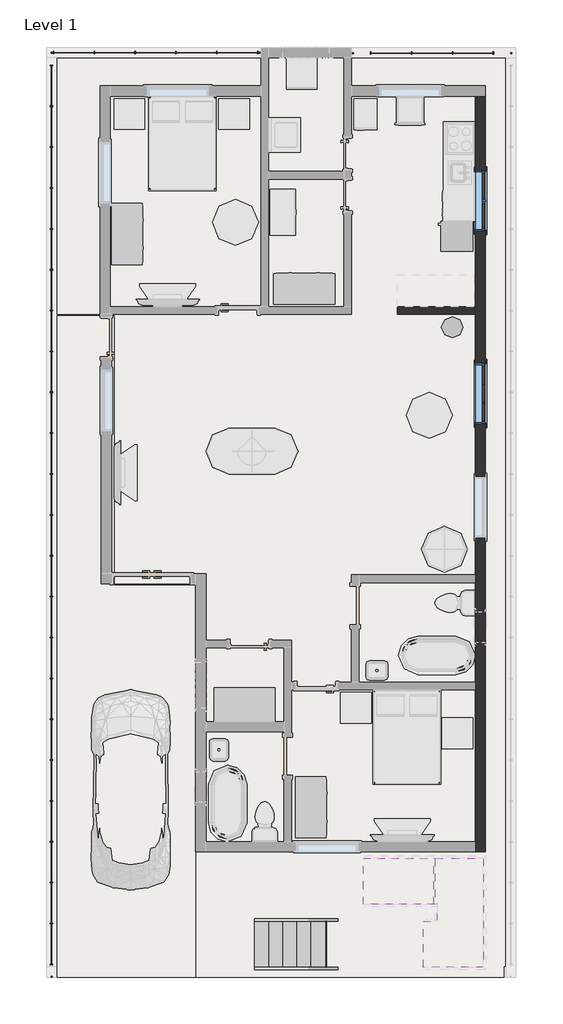
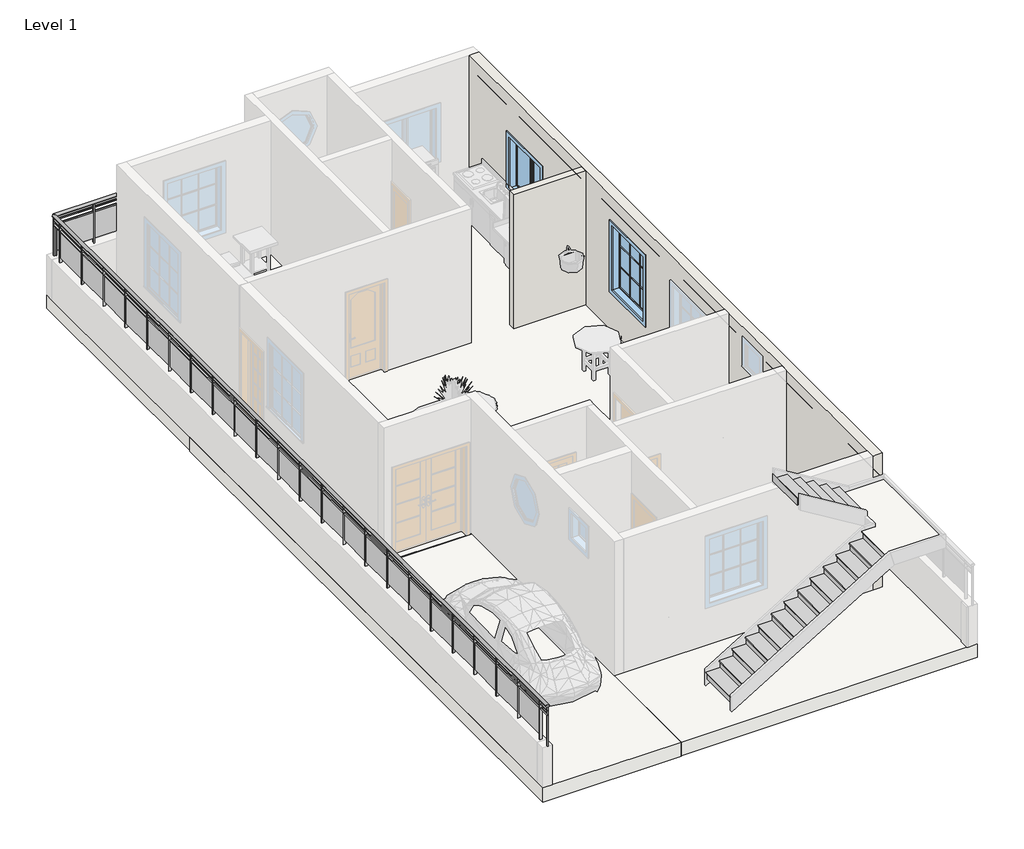
# One storey, part 2 of 3: 3 railings, 3 slabs, 2 stair flights, 2 walls, 2 windows.
"""IFC4 building model written with IfcOpenShell, lengths in millimetres."""

from ifc_helpers import new_model, si_unit, point, frame, origin, origin_with_axes, place, context, project, spatial, polyline, ellipse_curve, trimmed, outline, extrude, faceted_brep, transform, mapped, element, save
from ifc_brep_helpers import plane_surface, extruded_surface, advanced_brep
from components import non_monolithic_landing_d9a0f4c8, stair_flight_2c1cbba1, stair_flight_74d64587, window_cfa1ffdd, window_0862ab64

model = new_model("IFC4")

# Units and contexts
model_context = context("Model", 3, world=origin())
ifc_project = project(units=[si_unit("LENGTHUNIT", "METRE", prefix="MILLI")], contexts=[model_context])

# Site, building, storey
site = spatial("IfcSite", under=ifc_project)
building = spatial("IfcBuilding", under=site)
storey = spatial("IfcBuildingStorey", under=building, Name="Level 1", Elevation=0.0)

# Railings
placement = place(None, origin())
element("IfcRailing", 1, ObjectType="Glass Panel - Bottom Fill", at=placement, inside=storey, context=model_context, shape_type="SolidModel", body=[
    advanced_brep(
    [(-3535.608395, 15334.3151182, 1828.8), (-3535.608395, 15410.5151182, 1828.8), (-7675.808395, 15334.3151182, 1828.8), (-7675.808395, 15410.5151182, 1828.8)],
    [
        (0, 1, ellipse_curve(frame((-3535.608395, 15372.4151182, 1828.8), z_axis=(1.0, 0.0, 0.0), x_axis=(0.0, 1.0, 0.0)), 38.1, 28.575)),
        (1, 0, ellipse_curve(frame((-3535.608395, 15372.4151182, 1828.8), z_axis=(1.0, 0.0, 0.0), x_axis=(0.0, 1.0, 0.0)), 38.1, 28.575)),
        (2, 3, ellipse_curve(frame((-7675.808395, 15372.4151182, 1828.8), z_axis=(-1.0, 0.0, 0.0), x_axis=(0.0, 1.0, 0.0)), 38.1, 28.575)),
        (3, 2, ellipse_curve(frame((-7675.808395, 15372.4151182, 1828.8), z_axis=(-1.0, 0.0, 0.0), x_axis=(0.0, 1.0, 0.0)), 38.1, 28.575)),
        (0, 2),
        (3, 1),
    ],
    [
        plane_surface(frame((-3535.608395, 15372.4151182, 1828.8), z_axis=(1.0, 0.0, 0.0), x_axis=(0.0, -1.0, 0.0))),
        plane_surface(frame((-7675.808395, 15372.4151182, 1828.8), z_axis=(-1.0, 0.0, 0.0), x_axis=(0.0, -1.0, 0.0))),
        extruded_surface(trimmed(ellipse_curve(frame((-7675.808395, 15372.4151182, 1828.8), z_axis=(1.0, 0.0, 0.0), x_axis=(0.0, 1.0, 0.0)), 38.1, 28.575), [point((-7675.808395, 15334.3151182, 1828.8))], [point((-7675.808395, 15410.5151182, 1828.8))], True, "CARTESIAN"), (4140.2, 0.0, 0.0), 4140.2),
        extruded_surface(trimmed(ellipse_curve(frame((-7675.808395, 15372.4151182, 1828.8), z_axis=(1.0, 0.0, 0.0), x_axis=(0.0, 1.0, 0.0)), 38.1, 28.575), [point((-7675.808395, 15410.5151182, 1828.8))], [point((-7675.808395, 15334.3151182, 1828.8))], True, "CARTESIAN"), (4140.2, 0.0, 0.0), 4140.2),
    ],
    [
        (0, [[1, 2]]),
        (1, [[3, 4]]),
        (2, [[-1, 5, -4, 6]]),
        (3, [[-2, -6, -3, -5]]),
    ],
),
    extrude(outline(polyline([(-3535.608395, 15385.1151182), (-3535.608395, 15359.7151182), (-7675.808395, 15359.7151182), (-7675.808395, 15385.1151182), (-3535.608395, 15385.1151182)])), frame((0.0, 0.0, 1714.5), z_axis=(0.0, 0.0, 1.0), x_axis=(1.0, 0.0, 0.0)), (0.0, 0.0, 1.0), 25.4),
    extrude(outline(polyline([(-3535.608395, 15385.1151182), (-3535.608395, 15359.7151182), (-7675.808395, 15359.7151182), (-7675.808395, 15385.1151182), (-3535.608395, 15385.1151182)])), frame((0.0, 0.0, 1612.9), z_axis=(0.0, 0.0, 1.0), x_axis=(1.0, 0.0, 0.0)), (0.0, 0.0, 1.0), 25.4),
    extrude(outline(polyline([(-7631.358395, 15397.8151182), (-7631.358395, 15347.0151182), (-7644.058395, 15347.0151182), (-7644.058395, 15397.8151182), (-7631.358395, 15397.8151182)])), frame((0.0, 0.0, 914.4), z_axis=(0.0, 0.0, 1.0), x_axis=(1.0, 0.0, 0.0)), (0.0, 0.0, 1.0), 885.6788223),
    extrude(outline(polyline([(-6824.908395, 15365.8799612), (-7637.708395, 15365.8799612), (-7637.708395, 15372.2299612), (-6824.908395, 15372.2299612), (-6824.908395, 15365.8799612)])), frame((0.0, 0.0, 1016.0), z_axis=(0.0, 0.0, 1.0), x_axis=(1.0, 0.0, 0.0)), (0.0, 0.0, 1.0), 596.9),
    extrude(outline(polyline([(-6818.558395, 15397.8151182), (-6818.558395, 15347.0151182), (-6831.258395, 15347.0151182), (-6831.258395, 15397.8151182), (-6818.558395, 15397.8151182)])), frame((0.0, 0.0, 914.4), z_axis=(0.0, 0.0, 1.0), x_axis=(1.0, 0.0, 0.0)), (0.0, 0.0, 1.0), 885.6788223),
    extrude(outline(polyline([(-6012.108395, 15365.8799612), (-6824.908395, 15365.8799612), (-6824.908395, 15372.2299612), (-6012.108395, 15372.2299612), (-6012.108395, 15365.8799612)])), frame((0.0, 0.0, 1016.0), z_axis=(0.0, 0.0, 1.0), x_axis=(1.0, 0.0, 0.0)), (0.0, 0.0, 1.0), 596.9),
    extrude(outline(polyline([(-6005.758395, 15397.8151182), (-6005.758395, 15347.0151182), (-6018.458395, 15347.0151182), (-6018.458395, 15397.8151182), (-6005.758395, 15397.8151182)])), frame((0.0, 0.0, 914.4), z_axis=(0.0, 0.0, 1.0), x_axis=(1.0, 0.0, 0.0)), (0.0, 0.0, 1.0), 885.6788223),
    extrude(outline(polyline([(-5199.308395, 15365.8799612), (-6012.108395, 15365.8799612), (-6012.108395, 15372.2299612), (-5199.308395, 15372.2299612), (-5199.308395, 15365.8799612)])), frame((0.0, 0.0, 1016.0), z_axis=(0.0, 0.0, 1.0), x_axis=(1.0, 0.0, 0.0)), (0.0, 0.0, 1.0), 596.9),
    extrude(outline(polyline([(-5192.958395, 15397.8151182), (-5192.958395, 15347.0151182), (-5205.658395, 15347.0151182), (-5205.658395, 15397.8151182), (-5192.958395, 15397.8151182)])), frame((0.0, 0.0, 914.4), z_axis=(0.0, 0.0, 1.0), x_axis=(1.0, 0.0, 0.0)), (0.0, 0.0, 1.0), 885.6788223),
    extrude(outline(polyline([(-4386.508395, 15365.8799612), (-5199.308395, 15365.8799612), (-5199.308395, 15372.2299612), (-4386.508395, 15372.2299612), (-4386.508395, 15365.8799612)])), frame((0.0, 0.0, 1016.0), z_axis=(0.0, 0.0, 1.0), x_axis=(1.0, 0.0, 0.0)), (0.0, 0.0, 1.0), 596.9),
    extrude(outline(polyline([(-4380.158395, 15397.8151182), (-4380.158395, 15347.0151182), (-4392.858395, 15347.0151182), (-4392.858395, 15397.8151182), (-4380.158395, 15397.8151182)])), frame((0.0, 0.0, 914.4), z_axis=(0.0, 0.0, 1.0), x_axis=(1.0, 0.0, 0.0)), (0.0, 0.0, 1.0), 885.6788223),
    extrude(outline(polyline([(-3573.708395, 15365.8799612), (-4386.508395, 15365.8799612), (-4386.508395, 15372.2299612), (-3573.708395, 15372.2299612), (-3573.708395, 15365.8799612)])), frame((0.0, 0.0, 1016.0), z_axis=(0.0, 0.0, 1.0), x_axis=(1.0, 0.0, 0.0)), (0.0, 0.0, 1.0), 596.9),
    extrude(outline(polyline([(-3567.358395, 15397.8151182), (-3567.358395, 15347.0151182), (-3580.058395, 15347.0151182), (-3580.058395, 15397.8151182), (-3567.358395, 15397.8151182)])), frame((0.0, 0.0, 914.4), z_axis=(0.0, 0.0, 1.0), x_axis=(1.0, 0.0, 0.0)), (0.0, 0.0, 1.0), 885.6788223),
    extrude(outline(polyline([(-7663.108395, 15381.9401182), (-7663.108395, 15362.8901182), (-7682.158395, 15362.8901182), (-7682.158395, 15381.9401182), (-7663.108395, 15381.9401182)])), frame((0.0, 0.0, 914.4), z_axis=(0.0, 0.0, 1.0), x_axis=(1.0, 0.0, 0.0)), (0.0, 0.0, 1.0), 885.6788223),
    extrude(outline(polyline([(-3529.258395, 15381.9401182), (-3529.258395, 15362.8901182), (-3548.308395, 15362.8901182), (-3548.308395, 15381.9401182), (-3529.258395, 15381.9401182)])), frame((0.0, 0.0, 914.4), z_axis=(0.0, 0.0, 1.0), x_axis=(1.0, 0.0, 0.0)), (0.0, 0.0, 1.0), 885.6788223),
])
element("IfcRailing", 2, ObjectType="Glass Panel - Bottom Fill", at=placement, inside=storey, context=model_context, shape_type="SolidModel", body=[
    advanced_brep(
    [(-7637.708395, 15372.4151182, 1828.8), (-7713.908395, 15372.4151182, 1828.8), (-7637.708395, -3017.1848818, 1828.8), (-7713.908395, -3017.1848818, 1828.8)],
    [
        (0, 1, ellipse_curve(frame((-7675.808395, 15372.4151182, 1828.8), z_axis=(0.0, 1.0, 0.0), x_axis=(-1.0, 0.0, 0.0)), 38.1, 28.575)),
        (1, 0, ellipse_curve(frame((-7675.808395, 15372.4151182, 1828.8), z_axis=(0.0, 1.0, 0.0), x_axis=(-1.0, 0.0, 0.0)), 38.1, 28.575)),
        (2, 3, ellipse_curve(frame((-7675.808395, -3017.1848818, 1828.8), z_axis=(0.0, -1.0, 0.0), x_axis=(-1.0, 0.0, 0.0)), 38.1, 28.575)),
        (3, 2, ellipse_curve(frame((-7675.808395, -3017.1848818, 1828.8), z_axis=(0.0, -1.0, 0.0), x_axis=(-1.0, 0.0, 0.0)), 38.1, 28.575)),
        (0, 2),
        (3, 1),
    ],
    [
        plane_surface(frame((-7675.808395, 15372.4151182, 1828.8), z_axis=(0.0, 1.0, 0.0), x_axis=(0.0, 0.0, -1.0))),
        plane_surface(frame((-7675.808395, -3017.1848818, 1828.8), z_axis=(0.0, -1.0, 0.0), x_axis=(0.0, 0.0, -1.0))),
        extruded_surface(trimmed(ellipse_curve(frame((-7675.808395, -3017.1848818, 1828.8), z_axis=(0.0, 1.0, 0.0), x_axis=(-1.0, 0.0, 0.0)), 38.1, 28.575), [point((-7637.708395, -3017.1848818, 1828.8))], [point((-7713.908395, -3017.1848818, 1828.8))], True, "CARTESIAN"), (0.0, 18389.6, 0.0), 18389.6),
        extruded_surface(trimmed(ellipse_curve(frame((-7675.808395, -3017.1848818, 1828.8), z_axis=(0.0, 1.0, 0.0), x_axis=(-1.0, 0.0, 0.0)), 38.1, 28.575), [point((-7713.908395, -3017.1848818, 1828.8))], [point((-7637.708395, -3017.1848818, 1828.8))], True, "CARTESIAN"), (0.0, 18389.6, 0.0), 18389.6),
    ],
    [
        (0, [[1, 2]]),
        (1, [[3, 4]]),
        (2, [[-1, 5, -4, 6]]),
        (3, [[-2, -6, -3, -5]]),
    ],
),
    extrude(outline(polyline([(-7688.508395, 15372.4151182), (-7663.108395, 15372.4151182), (-7663.108395, -3017.1848818), (-7688.508395, -3017.1848818), (-7688.508395, 15372.4151182)])), frame((0.0, 0.0, 1714.5), z_axis=(0.0, 0.0, 1.0), x_axis=(1.0, 0.0, 0.0)), (0.0, 0.0, 1.0), 25.4),
    extrude(outline(polyline([(-7688.508395, 15372.4151182), (-7663.108395, 15372.4151182), (-7663.108395, -3017.1848818), (-7688.508395, -3017.1848818), (-7688.508395, 15372.4151182)])), frame((0.0, 0.0, 1612.9), z_axis=(0.0, 0.0, 1.0), x_axis=(1.0, 0.0, 0.0)), (0.0, 0.0, 1.0), 25.4),
    extrude(outline(polyline([(-7650.408395, -2756.8348818), (-7650.408395, -2769.5348818), (-7701.208395, -2769.5348818), (-7701.208395, -2756.8348818), (-7650.408395, -2756.8348818)])), frame((0.0, 0.0, 914.4), z_axis=(0.0, 0.0, 1.0), x_axis=(1.0, 0.0, 0.0)), (0.0, 0.0, 1.0), 885.6788223),
    extrude(outline(polyline([(-7682.343552, -1950.3848818), (-7675.993552, -1950.3848818), (-7675.993552, -2763.1848818), (-7682.343552, -2763.1848818), (-7682.343552, -1950.3848818)])), frame((0.0, 0.0, 1016.0), z_axis=(0.0, 0.0, 1.0), x_axis=(1.0, 0.0, 0.0)), (0.0, 0.0, 1.0), 596.9),
    extrude(outline(polyline([(-7650.408395, -1944.0348818), (-7650.408395, -1956.7348818), (-7701.208395, -1956.7348818), (-7701.208395, -1944.0348818), (-7650.408395, -1944.0348818)])), frame((0.0, 0.0, 914.4), z_axis=(0.0, 0.0, 1.0), x_axis=(1.0, 0.0, 0.0)), (0.0, 0.0, 1.0), 885.6788223),
    extrude(outline(polyline([(-7682.343552, -1137.5848818), (-7675.993552, -1137.5848818), (-7675.993552, -1950.3848818), (-7682.343552, -1950.3848818), (-7682.343552, -1137.5848818)])), frame((0.0, 0.0, 1016.0), z_axis=(0.0, 0.0, 1.0), x_axis=(1.0, 0.0, 0.0)), (0.0, 0.0, 1.0), 596.9),
    extrude(outline(polyline([(-7650.408395, -1131.2348818), (-7650.408395, -1143.9348818), (-7701.208395, -1143.9348818), (-7701.208395, -1131.2348818), (-7650.408395, -1131.2348818)])), frame((0.0, 0.0, 914.4), z_axis=(0.0, 0.0, 1.0), x_axis=(1.0, 0.0, 0.0)), (0.0, 0.0, 1.0), 885.6788223),
    extrude(outline(polyline([(-7682.343552, -324.7848818), (-7675.993552, -324.7848818), (-7675.993552, -1137.5848818), (-7682.343552, -1137.5848818), (-7682.343552, -324.7848818)])), frame((0.0, 0.0, 1016.0), z_axis=(0.0, 0.0, 1.0), x_axis=(1.0, 0.0, 0.0)), (0.0, 0.0, 1.0), 596.9),
    extrude(outline(polyline([(-7650.408395, -318.4348818), (-7650.408395, -331.1348818), (-7701.208395, -331.1348818), (-7701.208395, -318.4348818), (-7650.408395, -318.4348818)])), frame((0.0, 0.0, 914.4), z_axis=(0.0, 0.0, 1.0), x_axis=(1.0, 0.0, 0.0)), (0.0, 0.0, 1.0), 885.6788223),
    extrude(outline(polyline([(-7682.343552, 488.0151182), (-7675.993552, 488.0151182), (-7675.993552, -324.7848818), (-7682.343552, -324.7848818), (-7682.343552, 488.0151182)])), frame((0.0, 0.0, 1016.0), z_axis=(0.0, 0.0, 1.0), x_axis=(1.0, 0.0, 0.0)), (0.0, 0.0, 1.0), 596.9),
    extrude(outline(polyline([(-7650.408395, 494.3651182), (-7650.408395, 481.6651182), (-7701.208395, 481.6651182), (-7701.208395, 494.3651182), (-7650.408395, 494.3651182)])), frame((0.0, 0.0, 914.4), z_axis=(0.0, 0.0, 1.0), x_axis=(1.0, 0.0, 0.0)), (0.0, 0.0, 1.0), 885.6788223),
    extrude(outline(polyline([(-7682.343552, 1300.8151182), (-7675.993552, 1300.8151182), (-7675.993552, 488.0151182), (-7682.343552, 488.0151182), (-7682.343552, 1300.8151182)])), frame((0.0, 0.0, 1016.0), z_axis=(0.0, 0.0, 1.0), x_axis=(1.0, 0.0, 0.0)), (0.0, 0.0, 1.0), 596.9),
    extrude(outline(polyline([(-7650.408395, 1307.1651182), (-7650.408395, 1294.4651182), (-7701.208395, 1294.4651182), (-7701.208395, 1307.1651182), (-7650.408395, 1307.1651182)])), frame((0.0, 0.0, 914.4), z_axis=(0.0, 0.0, 1.0), x_axis=(1.0, 0.0, 0.0)), (0.0, 0.0, 1.0), 885.6788223),
    extrude(outline(polyline([(-7682.343552, 2113.6151182), (-7675.993552, 2113.6151182), (-7675.993552, 1300.8151182), (-7682.343552, 1300.8151182), (-7682.343552, 2113.6151182)])), frame((0.0, 0.0, 1016.0), z_axis=(0.0, 0.0, 1.0), x_axis=(1.0, 0.0, 0.0)), (0.0, 0.0, 1.0), 596.9),
    extrude(outline(polyline([(-7650.408395, 2119.9651182), (-7650.408395, 2107.2651182), (-7701.208395, 2107.2651182), (-7701.208395, 2119.9651182), (-7650.408395, 2119.9651182)])), frame((0.0, 0.0, 914.4), z_axis=(0.0, 0.0, 1.0), x_axis=(1.0, 0.0, 0.0)), (0.0, 0.0, 1.0), 885.6788223),
    extrude(outline(polyline([(-7682.343552, 2926.4151182), (-7675.993552, 2926.4151182), (-7675.993552, 2113.6151182), (-7682.343552, 2113.6151182), (-7682.343552, 2926.4151182)])), frame((0.0, 0.0, 1016.0), z_axis=(0.0, 0.0, 1.0), x_axis=(1.0, 0.0, 0.0)), (0.0, 0.0, 1.0), 596.9),
    extrude(outline(polyline([(-7650.408395, 2932.7651182), (-7650.408395, 2920.0651182), (-7701.208395, 2920.0651182), (-7701.208395, 2932.7651182), (-7650.408395, 2932.7651182)])), frame((0.0, 0.0, 914.4), z_axis=(0.0, 0.0, 1.0), x_axis=(1.0, 0.0, 0.0)), (0.0, 0.0, 1.0), 885.6788223),
    extrude(outline(polyline([(-7682.343552, 3739.2151182), (-7675.993552, 3739.2151182), (-7675.993552, 2926.4151182), (-7682.343552, 2926.4151182), (-7682.343552, 3739.2151182)])), frame((0.0, 0.0, 1016.0), z_axis=(0.0, 0.0, 1.0), x_axis=(1.0, 0.0, 0.0)), (0.0, 0.0, 1.0), 596.9),
    extrude(outline(polyline([(-7650.408395, 3745.5651182), (-7650.408395, 3732.8651182), (-7701.208395, 3732.8651182), (-7701.208395, 3745.5651182), (-7650.408395, 3745.5651182)])), frame((0.0, 0.0, 914.4), z_axis=(0.0, 0.0, 1.0), x_axis=(1.0, 0.0, 0.0)), (0.0, 0.0, 1.0), 885.6788223),
    extrude(outline(polyline([(-7682.343552, 4552.0151182), (-7675.993552, 4552.0151182), (-7675.993552, 3739.2151182), (-7682.343552, 3739.2151182), (-7682.343552, 4552.0151182)])), frame((0.0, 0.0, 1016.0), z_axis=(0.0, 0.0, 1.0), x_axis=(1.0, 0.0, 0.0)), (0.0, 0.0, 1.0), 596.9),
    extrude(outline(polyline([(-7650.408395, 4558.3651182), (-7650.408395, 4545.6651182), (-7701.208395, 4545.6651182), (-7701.208395, 4558.3651182), (-7650.408395, 4558.3651182)])), frame((0.0, 0.0, 914.4), z_axis=(0.0, 0.0, 1.0), x_axis=(1.0, 0.0, 0.0)), (0.0, 0.0, 1.0), 885.6788223),
    extrude(outline(polyline([(-7682.343552, 5364.8151182), (-7675.993552, 5364.8151182), (-7675.993552, 4552.0151182), (-7682.343552, 4552.0151182), (-7682.343552, 5364.8151182)])), frame((0.0, 0.0, 1016.0), z_axis=(0.0, 0.0, 1.0), x_axis=(1.0, 0.0, 0.0)), (0.0, 0.0, 1.0), 596.9),
    extrude(outline(polyline([(-7650.408395, 5371.1651182), (-7650.408395, 5358.4651182), (-7701.208395, 5358.4651182), (-7701.208395, 5371.1651182), (-7650.408395, 5371.1651182)])), frame((0.0, 0.0, 914.4), z_axis=(0.0, 0.0, 1.0), x_axis=(1.0, 0.0, 0.0)), (0.0, 0.0, 1.0), 885.6788223),
    extrude(outline(polyline([(-7682.343552, 6177.6151182), (-7675.993552, 6177.6151182), (-7675.993552, 5364.8151182), (-7682.343552, 5364.8151182), (-7682.343552, 6177.6151182)])), frame((0.0, 0.0, 1016.0), z_axis=(0.0, 0.0, 1.0), x_axis=(1.0, 0.0, 0.0)), (0.0, 0.0, 1.0), 596.9),
    extrude(outline(polyline([(-7650.408395, 6183.9651182), (-7650.408395, 6171.2651182), (-7701.208395, 6171.2651182), (-7701.208395, 6183.9651182), (-7650.408395, 6183.9651182)])), frame((0.0, 0.0, 914.4), z_axis=(0.0, 0.0, 1.0), x_axis=(1.0, 0.0, 0.0)), (0.0, 0.0, 1.0), 885.6788223),
    extrude(outline(polyline([(-7682.343552, 6990.4151182), (-7675.993552, 6990.4151182), (-7675.993552, 6177.6151182), (-7682.343552, 6177.6151182), (-7682.343552, 6990.4151182)])), frame((0.0, 0.0, 1016.0), z_axis=(0.0, 0.0, 1.0), x_axis=(1.0, 0.0, 0.0)), (0.0, 0.0, 1.0), 596.9),
    extrude(outline(polyline([(-7650.408395, 6996.7651182), (-7650.408395, 6984.0651182), (-7701.208395, 6984.0651182), (-7701.208395, 6996.7651182), (-7650.408395, 6996.7651182)])), frame((0.0, 0.0, 914.4), z_axis=(0.0, 0.0, 1.0), x_axis=(1.0, 0.0, 0.0)), (0.0, 0.0, 1.0), 885.6788223),
    extrude(outline(polyline([(-7682.343552, 7803.2151182), (-7675.993552, 7803.2151182), (-7675.993552, 6990.4151182), (-7682.343552, 6990.4151182), (-7682.343552, 7803.2151182)])), frame((0.0, 0.0, 1016.0), z_axis=(0.0, 0.0, 1.0), x_axis=(1.0, 0.0, 0.0)), (0.0, 0.0, 1.0), 596.9),
    extrude(outline(polyline([(-7650.408395, 7809.5651182), (-7650.408395, 7796.8651182), (-7701.208395, 7796.8651182), (-7701.208395, 7809.5651182), (-7650.408395, 7809.5651182)])), frame((0.0, 0.0, 914.4), z_axis=(0.0, 0.0, 1.0), x_axis=(1.0, 0.0, 0.0)), (0.0, 0.0, 1.0), 885.6788223),
    extrude(outline(polyline([(-7682.343552, 8616.0151182), (-7675.993552, 8616.0151182), (-7675.993552, 7803.2151182), (-7682.343552, 7803.2151182), (-7682.343552, 8616.0151182)])), frame((0.0, 0.0, 1016.0), z_axis=(0.0, 0.0, 1.0), x_axis=(1.0, 0.0, 0.0)), (0.0, 0.0, 1.0), 596.9),
    extrude(outline(polyline([(-7650.408395, 8622.3651182), (-7650.408395, 8609.6651182), (-7701.208395, 8609.6651182), (-7701.208395, 8622.3651182), (-7650.408395, 8622.3651182)])), frame((0.0, 0.0, 914.4), z_axis=(0.0, 0.0, 1.0), x_axis=(1.0, 0.0, 0.0)), (0.0, 0.0, 1.0), 885.6788223),
    extrude(outline(polyline([(-7682.343552, 9428.8151182), (-7675.993552, 9428.8151182), (-7675.993552, 8616.0151182), (-7682.343552, 8616.0151182), (-7682.343552, 9428.8151182)])), frame((0.0, 0.0, 1016.0), z_axis=(0.0, 0.0, 1.0), x_axis=(1.0, 0.0, 0.0)), (0.0, 0.0, 1.0), 596.9),
    extrude(outline(polyline([(-7650.408395, 9435.1651182), (-7650.408395, 9422.4651182), (-7701.208395, 9422.4651182), (-7701.208395, 9435.1651182), (-7650.408395, 9435.1651182)])), frame((0.0, 0.0, 914.4), z_axis=(0.0, 0.0, 1.0), x_axis=(1.0, 0.0, 0.0)), (0.0, 0.0, 1.0), 885.6788223),
    extrude(outline(polyline([(-7682.343552, 10241.6151182), (-7675.993552, 10241.6151182), (-7675.993552, 9428.8151182), (-7682.343552, 9428.8151182), (-7682.343552, 10241.6151182)])), frame((0.0, 0.0, 1016.0), z_axis=(0.0, 0.0, 1.0), x_axis=(1.0, 0.0, 0.0)), (0.0, 0.0, 1.0), 596.9),
    extrude(outline(polyline([(-7650.408395, 10247.9651182), (-7650.408395, 10235.2651182), (-7701.208395, 10235.2651182), (-7701.208395, 10247.9651182), (-7650.408395, 10247.9651182)])), frame((0.0, 0.0, 914.4), z_axis=(0.0, 0.0, 1.0), x_axis=(1.0, 0.0, 0.0)), (0.0, 0.0, 1.0), 885.6788223),
    extrude(outline(polyline([(-7682.343552, 11054.4151182), (-7675.993552, 11054.4151182), (-7675.993552, 10241.6151182), (-7682.343552, 10241.6151182), (-7682.343552, 11054.4151182)])), frame((0.0, 0.0, 1016.0), z_axis=(0.0, 0.0, 1.0), x_axis=(1.0, 0.0, 0.0)), (0.0, 0.0, 1.0), 596.9),
    extrude(outline(polyline([(-7650.408395, 11060.7651182), (-7650.408395, 11048.0651182), (-7701.208395, 11048.0651182), (-7701.208395, 11060.7651182), (-7650.408395, 11060.7651182)])), frame((0.0, 0.0, 914.4), z_axis=(0.0, 0.0, 1.0), x_axis=(1.0, 0.0, 0.0)), (0.0, 0.0, 1.0), 885.6788223),
    extrude(outline(polyline([(-7682.343552, 11867.2151182), (-7675.993552, 11867.2151182), (-7675.993552, 11054.4151182), (-7682.343552, 11054.4151182), (-7682.343552, 11867.2151182)])), frame((0.0, 0.0, 1016.0), z_axis=(0.0, 0.0, 1.0), x_axis=(1.0, 0.0, 0.0)), (0.0, 0.0, 1.0), 596.9),
    extrude(outline(polyline([(-7650.408395, 11873.5651182), (-7650.408395, 11860.8651182), (-7701.208395, 11860.8651182), (-7701.208395, 11873.5651182), (-7650.408395, 11873.5651182)])), frame((0.0, 0.0, 914.4), z_axis=(0.0, 0.0, 1.0), x_axis=(1.0, 0.0, 0.0)), (0.0, 0.0, 1.0), 885.6788223),
    extrude(outline(polyline([(-7682.343552, 12680.0151182), (-7675.993552, 12680.0151182), (-7675.993552, 11867.2151182), (-7682.343552, 11867.2151182), (-7682.343552, 12680.0151182)])), frame((0.0, 0.0, 1016.0), z_axis=(0.0, 0.0, 1.0), x_axis=(1.0, 0.0, 0.0)), (0.0, 0.0, 1.0), 596.9),
    extrude(outline(polyline([(-7650.408395, 12686.3651182), (-7650.408395, 12673.6651182), (-7701.208395, 12673.6651182), (-7701.208395, 12686.3651182), (-7650.408395, 12686.3651182)])), frame((0.0, 0.0, 914.4), z_axis=(0.0, 0.0, 1.0), x_axis=(1.0, 0.0, 0.0)), (0.0, 0.0, 1.0), 885.6788223),
    extrude(outline(polyline([(-7682.343552, 13492.8151182), (-7675.993552, 13492.8151182), (-7675.993552, 12680.0151182), (-7682.343552, 12680.0151182), (-7682.343552, 13492.8151182)])), frame((0.0, 0.0, 1016.0), z_axis=(0.0, 0.0, 1.0), x_axis=(1.0, 0.0, 0.0)), (0.0, 0.0, 1.0), 596.9),
    extrude(outline(polyline([(-7650.408395, 13499.1651182), (-7650.408395, 13486.4651182), (-7701.208395, 13486.4651182), (-7701.208395, 13499.1651182), (-7650.408395, 13499.1651182)])), frame((0.0, 0.0, 914.4), z_axis=(0.0, 0.0, 1.0), x_axis=(1.0, 0.0, 0.0)), (0.0, 0.0, 1.0), 885.6788223),
    extrude(outline(polyline([(-7682.343552, 14305.6151182), (-7675.993552, 14305.6151182), (-7675.993552, 13492.8151182), (-7682.343552, 13492.8151182), (-7682.343552, 14305.6151182)])), frame((0.0, 0.0, 1016.0), z_axis=(0.0, 0.0, 1.0), x_axis=(1.0, 0.0, 0.0)), (0.0, 0.0, 1.0), 596.9),
    extrude(outline(polyline([(-7650.408395, 14311.9651182), (-7650.408395, 14299.2651182), (-7701.208395, 14299.2651182), (-7701.208395, 14311.9651182), (-7650.408395, 14311.9651182)])), frame((0.0, 0.0, 914.4), z_axis=(0.0, 0.0, 1.0), x_axis=(1.0, 0.0, 0.0)), (0.0, 0.0, 1.0), 885.6788223),
    extrude(outline(polyline([(-7682.343552, 15118.4151182), (-7675.993552, 15118.4151182), (-7675.993552, 14305.6151182), (-7682.343552, 14305.6151182), (-7682.343552, 15118.4151182)])), frame((0.0, 0.0, 1016.0), z_axis=(0.0, 0.0, 1.0), x_axis=(1.0, 0.0, 0.0)), (0.0, 0.0, 1.0), 596.9),
    extrude(outline(polyline([(-7650.408395, 15124.7651182), (-7650.408395, 15112.0651182), (-7701.208395, 15112.0651182), (-7701.208395, 15124.7651182), (-7650.408395, 15124.7651182)])), frame((0.0, 0.0, 914.4), z_axis=(0.0, 0.0, 1.0), x_axis=(1.0, 0.0, 0.0)), (0.0, 0.0, 1.0), 885.6788223),
    extrude(outline(polyline([(-7666.283395, -3004.4848818), (-7666.283395, -3023.5348818), (-7685.333395, -3023.5348818), (-7685.333395, -3004.4848818), (-7666.283395, -3004.4848818)])), frame((0.0, 0.0, 914.4), z_axis=(0.0, 0.0, 1.0), x_axis=(1.0, 0.0, 0.0)), (0.0, 0.0, 1.0), 885.6788223),
    extrude(outline(polyline([(-7666.283395, 15378.7651182), (-7666.283395, 15359.7151182), (-7685.333395, 15359.7151182), (-7685.333395, 15378.7651182), (-7666.283395, 15378.7651182)])), frame((0.0, 0.0, 914.4), z_axis=(0.0, 0.0, 1.0), x_axis=(1.0, 0.0, 0.0)), (0.0, 0.0, 1.0), 885.6788223),
])
element("IfcRailing", 3, ObjectType="Glass Panel - Bottom Fill", at=placement, inside=storey, context=model_context, shape_type="SolidModel", body=[
    advanced_brep(
    [(1477.716605, 15324.7901182, 1828.8), (1477.716605, 15400.9901182, 1828.8), (-1681.408395, 15324.7901182, 1828.8), (-1681.408395, 15400.9901182, 1828.8)],
    [
        (0, 1, ellipse_curve(frame((1477.716605, 15362.8901182, 1828.8), z_axis=(1.0, 0.0, 0.0), x_axis=(0.0, 1.0, 0.0)), 38.1, 28.575)),
        (1, 0, ellipse_curve(frame((1477.716605, 15362.8901182, 1828.8), z_axis=(1.0, 0.0, 0.0), x_axis=(0.0, 1.0, 0.0)), 38.1, 28.575)),
        (2, 3, ellipse_curve(frame((-1681.408395, 15362.8901182, 1828.8), z_axis=(-1.0, 0.0, 0.0), x_axis=(0.0, 1.0, 0.0)), 38.1, 28.575)),
        (3, 2, ellipse_curve(frame((-1681.408395, 15362.8901182, 1828.8), z_axis=(-1.0, 0.0, 0.0), x_axis=(0.0, 1.0, 0.0)), 38.1, 28.575)),
        (0, 2),
        (3, 1),
    ],
    [
        plane_surface(frame((1477.716605, 15362.8901182, 1828.8), z_axis=(1.0, 0.0, 0.0), x_axis=(0.0, -1.0, 0.0))),
        plane_surface(frame((-1681.408395, 15362.8901182, 1828.8), z_axis=(-1.0, 0.0, 0.0), x_axis=(0.0, -1.0, 0.0))),
        extruded_surface(trimmed(ellipse_curve(frame((-1681.408395, 15362.8901182, 1828.8), z_axis=(1.0, 0.0, 0.0), x_axis=(0.0, 1.0, 0.0)), 38.1, 28.575), [point((-1681.408395, 15324.7901182, 1828.8))], [point((-1681.408395, 15400.9901182, 1828.8))], True, "CARTESIAN"), (3159.125, 0.0, 0.0), 3159.125),
        extruded_surface(trimmed(ellipse_curve(frame((-1681.408395, 15362.8901182, 1828.8), z_axis=(1.0, 0.0, 0.0), x_axis=(0.0, 1.0, 0.0)), 38.1, 28.575), [point((-1681.408395, 15400.9901182, 1828.8))], [point((-1681.408395, 15324.7901182, 1828.8))], True, "CARTESIAN"), (3159.125, 0.0, 0.0), 3159.125),
    ],
    [
        (0, [[1, 2]]),
        (1, [[3, 4]]),
        (2, [[-1, 5, -4, 6]]),
        (3, [[-2, -6, -3, -5]]),
    ],
),
    extrude(outline(polyline([(1477.716605, 15375.5901182), (1477.716605, 15350.1901182), (-1681.408395, 15350.1901182), (-1681.408395, 15375.5901182), (1477.716605, 15375.5901182)])), frame((0.0, 0.0, 1714.5), z_axis=(0.0, 0.0, 1.0), x_axis=(1.0, 0.0, 0.0)), (0.0, 0.0, 1.0), 25.4),
    extrude(outline(polyline([(1477.716605, 15375.5901182), (1477.716605, 15350.1901182), (-1681.408395, 15350.1901182), (-1681.408395, 15375.5901182), (1477.716605, 15375.5901182)])), frame((0.0, 0.0, 1612.9), z_axis=(0.0, 0.0, 1.0), x_axis=(1.0, 0.0, 0.0)), (0.0, 0.0, 1.0), 25.4),
    extrude(outline(polyline([(-1314.695895, 15388.2901182), (-1314.695895, 15337.4901182), (-1327.395895, 15337.4901182), (-1327.395895, 15388.2901182), (-1314.695895, 15388.2901182)])), frame((0.0, 0.0, 914.4), z_axis=(0.0, 0.0, 1.0), x_axis=(1.0, 0.0, 0.0)), (0.0, 0.0, 1.0), 885.6788223),
    extrude(outline(polyline([(-508.245895, 15356.3549612), (-1321.045895, 15356.3549612), (-1321.045895, 15362.7049612), (-508.245895, 15362.7049612), (-508.245895, 15356.3549612)])), frame((0.0, 0.0, 1016.0), z_axis=(0.0, 0.0, 1.0), x_axis=(1.0, 0.0, 0.0)), (0.0, 0.0, 1.0), 596.9),
    extrude(outline(polyline([(-501.895895, 15388.2901182), (-501.895895, 15337.4901182), (-514.595895, 15337.4901182), (-514.595895, 15388.2901182), (-501.895895, 15388.2901182)])), frame((0.0, 0.0, 914.4), z_axis=(0.0, 0.0, 1.0), x_axis=(1.0, 0.0, 0.0)), (0.0, 0.0, 1.0), 885.6788223),
    extrude(outline(polyline([(304.554105, 15356.3549612), (-508.245895, 15356.3549612), (-508.245895, 15362.7049612), (304.554105, 15362.7049612), (304.554105, 15356.3549612)])), frame((0.0, 0.0, 1016.0), z_axis=(0.0, 0.0, 1.0), x_axis=(1.0, 0.0, 0.0)), (0.0, 0.0, 1.0), 596.9),
    extrude(outline(polyline([(310.904105, 15388.2901182), (310.904105, 15337.4901182), (298.204105, 15337.4901182), (298.204105, 15388.2901182), (310.904105, 15388.2901182)])), frame((0.0, 0.0, 914.4), z_axis=(0.0, 0.0, 1.0), x_axis=(1.0, 0.0, 0.0)), (0.0, 0.0, 1.0), 885.6788223),
    extrude(outline(polyline([(1117.354105, 15356.3549612), (304.554105, 15356.3549612), (304.554105, 15362.7049612), (1117.354105, 15362.7049612), (1117.354105, 15356.3549612)])), frame((0.0, 0.0, 1016.0), z_axis=(0.0, 0.0, 1.0), x_axis=(1.0, 0.0, 0.0)), (0.0, 0.0, 1.0), 596.9),
    extrude(outline(polyline([(1123.704105, 15388.2901182), (1123.704105, 15337.4901182), (1111.004105, 15337.4901182), (1111.004105, 15388.2901182), (1123.704105, 15388.2901182)])), frame((0.0, 0.0, 914.4), z_axis=(0.0, 0.0, 1.0), x_axis=(1.0, 0.0, 0.0)), (0.0, 0.0, 1.0), 885.6788223),
    extrude(outline(polyline([(-1668.708395, 15372.4151182), (-1668.708395, 15353.3651182), (-1687.758395, 15353.3651182), (-1687.758395, 15372.4151182), (-1668.708395, 15372.4151182)])), frame((0.0, 0.0, 914.4), z_axis=(0.0, 0.0, 1.0), x_axis=(1.0, 0.0, 0.0)), (0.0, 0.0, 1.0), 885.6788223),
    extrude(outline(polyline([(1484.066605, 15372.4151182), (1484.066605, 15353.3651182), (1465.016605, 15353.3651182), (1465.016605, 15372.4151182), (1484.066605, 15372.4151182)])), frame((0.0, 0.0, 914.4), z_axis=(0.0, 0.0, 1.0), x_axis=(1.0, 0.0, 0.0)), (0.0, 0.0, 1.0), 885.6788223),
])

# Slabs
element("IfcSlab", 4, at=placement, inside=storey, context=model_context, shape_type="SweptSolid", body=[
    extrude(outline(polyline([(-6431.208395, 10140.0151182), (-6431.208395, 4780.6151182), (-4805.608395, 4780.6151182), (-4805.608395, -3017.1848818), (-7777.408395, -3017.1848818), (-7777.408395, 10140.0151182), (-6431.208395, 10140.0151182)])), frame((0.0, 0.0, -323.85), z_axis=(0.0, 0.0, 1.0), x_axis=(1.0, 0.0, 0.0)), (0.0, 0.0, 1.0), 323.85),
])
element("IfcSlab", 5, ObjectType="Generic - 12\" - Filled", at=placement, inside=storey, context=model_context, shape_type="SweptSolid", body=[
    extrude(outline(polyline([(1569.791605, 15474.0151182), (1569.791605, -3017.1848818), (-4805.608395, -3017.1848818), (-4805.608395, 4806.0151182), (-6685.208395, 4806.0151182), (-6685.208395, 10165.4151182), (-7777.408395, 10165.4151182), (-7777.408395, 15474.0151182), (1569.791605, 15474.0151182)])), frame((0.0, 0.0, -304.8), z_axis=(0.0, 0.0, 1.0), x_axis=(1.0, 0.0, 0.0)), (0.0, 0.0, 1.0), 304.8),
])
non_monolithic_landing_shape = non_monolithic_landing_d9a0f4c8(model_context)
element("IfcSlab", 6, ObjectType="Non-Monolithic Landing", at=placement, inside=storey, context=model_context, shape_type="MappedRepresentation", body=[
    mapped(non_monolithic_landing_shape, transform((0.0, 0.0, 0.0), x_axis=(1.0, 0.0, 0.0), y_axis=(0.0, 1.0, 0.0), z_axis=(0.0, 0.0, 1.0))),
])

# Stair flights
stair_flight_shape = stair_flight_2c1cbba1(model_context)
element("IfcStairFlight", 7, ObjectType="2\" Tread 1\" Nosing 1/4\" Riser", at=placement, inside=storey, context=model_context, shape_type="MappedRepresentation", body=[
    mapped(stair_flight_shape, transform((0.0, 0.0, 0.0), x_axis=(1.0, 0.0, 0.0), y_axis=(0.0, 1.0, 0.0), z_axis=(0.0, 0.0, 1.0))),
])
stair_flight_2_shape = stair_flight_74d64587(model_context)
element("IfcStairFlight", 8, ObjectType="2\" Tread 1\" Nosing 1/4\" Riser", at=placement, inside=storey, context=model_context, shape_type="MappedRepresentation", body=[
    mapped(stair_flight_2_shape, transform((0.0, 0.0, 0.0), x_axis=(1.0, 0.0, 0.0), y_axis=(0.0, 1.0, 0.0), z_axis=(0.0, 0.0, 1.0))),
])

# Walls
element("IfcWall", 9, ObjectType="Generic - 8\"", at=placement, inside=storey, context=model_context, shape_type="Brep", body=[
    faceted_brep([(756.991605, 14508.8151182, 0.0), (756.991605, 10317.8151182, 0.0), (756.991605, 10165.4151182, 0.0), (756.991605, 4983.8151182, 0.0), (756.991605, 4831.4151182, 0.0), (756.991605, 2850.2151182, 0.0), (756.991605, 2697.8151182, 0.0), (756.991605, -324.7848818, 0.0), (756.991605, -527.9848818, 0.0), (756.991605, -527.9848818, 3048.0), (756.991605, -324.7848818, 3048.0), (756.991605, 2697.8151182, 3048.0), (756.991605, 2850.2151182, 3048.0), (756.991605, 4831.4151182, 3048.0), (756.991605, 4983.8151182, 3048.0), (756.991605, 10165.4151182, 3048.0), (756.991605, 10317.8151182, 3048.0), (756.991605, 14508.8151182, 3048.0), (756.991605, 5720.4151182, 2438.4), (756.991605, 5720.4151182, 914.4), (756.991605, 6939.6151182, 914.4), (756.991605, 6939.6151182, 2438.4), (756.991605, 7981.0151182, 2438.4), (756.991605, 7981.0151182, 914.4), (756.991605, 9200.2151182, 914.4), (756.991605, 9200.2151182, 2438.4), (756.991605, 11816.4151182, 2133.6), (756.991605, 11816.4151182, 914.4), (756.991605, 13035.6151182, 914.4), (756.991605, 13035.6151182, 2133.6), (756.991605, 4247.2151182, 2768.6), (756.991605, 3637.6151182, 2768.6), (756.991605, 3637.6151182, 2159.0), (756.991605, 4247.2151182, 2159.0), (960.191605, 14508.8151182, 0.0), (960.191605, 14508.8151182, 3048.0), (960.191605, -527.9848818, 3048.0), (960.191605, -527.9848818, 0.0), (960.191605, 5720.4151182, 2438.4), (960.191605, 6939.6151182, 2438.4), (960.191605, 6939.6151182, 914.4), (960.191605, 5720.4151182, 914.4), (960.191605, 7981.0151182, 2438.4), (960.191605, 9200.2151182, 2438.4), (960.191605, 9200.2151182, 914.4), (960.191605, 7981.0151182, 914.4), (960.191605, 11816.4151182, 2133.6), (960.191605, 13035.6151182, 2133.6), (960.191605, 13035.6151182, 914.4), (960.191605, 11816.4151182, 914.4), (960.191605, 4247.2151182, 2768.6), (960.191605, 4247.2151182, 2159.0), (960.191605, 3637.6151182, 2159.0), (960.191605, 3637.6151182, 2768.6)], [[[0, 1, 2, 3, 4, 5, 6, 7, 8, 9, 10, 11, 12, 13, 14, 15, 16, 17], [18, 19, 20, 21], [22, 23, 24, 25], [26, 27, 28, 29], [30, 31, 32, 33]], [[34, 35, 36, 37], [38, 39, 40, 41], [42, 43, 44, 45], [46, 47, 48, 49], [50, 51, 52, 53]], [[8, 7, 6, 5, 4, 3, 2, 1, 0, 34, 37]], [[0, 17, 35, 34]], [[9, 8, 37, 36]], [[19, 18, 38, 41]], [[20, 19, 41, 40]], [[21, 20, 40, 39]], [[18, 21, 39, 38]], [[23, 22, 42, 45]], [[24, 23, 45, 44]], [[25, 24, 44, 43]], [[22, 25, 43, 42]], [[27, 26, 46, 49]], [[28, 27, 49, 48]], [[29, 28, 48, 47]], [[26, 29, 47, 46]], [[17, 16, 15, 14, 13, 12, 11, 10, 9, 36, 35]], [[51, 50, 30, 33]], [[52, 51, 33, 32]], [[53, 52, 32, 31]], [[50, 53, 31, 30]]]),
])
element("IfcWall", 10, ObjectType="INNER WALL", at=placement, inside=storey, context=model_context, shape_type="SweptSolid", body=[
    extrude(outline(polyline([(756.991605, 10165.4151182), (-792.408395, 10165.4151182), (-792.408395, 10317.8151182), (756.991605, 10317.8151182), (756.991605, 10165.4151182)])), origin_with_axes(), (0.0, 0.0, 1.0), 3048.0),
])

# Windows
window_shape = window_cfa1ffdd(model_context)
element("IfcWindow", 11, ObjectType="Casement 3x3 with Trim : 48\" x 60\"", at=placement, inside=storey, context=model_context, shape_type="MappedRepresentation", body=[
    mapped(window_shape, transform((858.591605, 8590.6151182, 304.8), x_axis=(0.0, -1.0, 0.0), y_axis=(1.0, 0.0, 0.0), z_axis=(0.0, 0.0, 1.0))),
])
window_2_shape = window_0862ab64(model_context)
element("IfcWindow", 12, ObjectType="Casement Dbl with Trim : 48\" x 48\"", at=placement, inside=storey, context=model_context, shape_type="MappedRepresentation", body=[
    mapped(window_2_shape, transform((839.541605, 12426.0151182, 0.0), x_axis=(0.0, -1.0, 0.0), y_axis=(1.0, 0.0, 0.0), z_axis=(0.0, 0.0, 1.0))),
])

save(model, "model.ifc")

# Revit data of these elements
# Type "Glass Panel - Bottom Fill"
#   Assembly Code = "C2010400"
#   built-in parameter 1008612 = 0.0416667 (stored number, unit not read)
#   built-in parameter 1008611 = 0.0416667 (stored number, unit not read)
#   built-in parameter 1008609 = 0.333333 (stored number, unit not read)
#   built-in parameter 1008604 = 0.166667 (stored number, unit not read)
#   built-in parameter 1008603 = 0.166667 (stored number, unit not read)
#   Railing Height = 3' - 0"
#   built-in parameter 1008630 = 2
#   built-in parameter 1008610 = 2
#   built-in parameter 1008618 = Baluster - Square : 3/4"
# Type
#   Assembly Code = "B1010"
#   Function = 0
#   Layers, outside or top first: 0' - 0 1/8" "Carpet (1)" (function 4); 0' - 0 3/4" "Plywood, Sheathing" (function 1); 0' - 11 7/8" "Structure, Wood Joist/Rafter Layer" (function 1)
# Type "Generic - 12\" - Filled"
#   Assembly Code = "B1010"
#   Function = 0
#   Layers, outside or top first: 1' - 0" no material (function 1)
# Type "Generic - 8\""
#   Assembly Code = "B2010"
#   Layers, outside or top first: 0' - 8" "Brick, Common" (function 1)
# Type "INNER WALL"
#   Assembly Code = "B2010"
#   Layers, outside or top first: 0' - 6" "Brick, Common" (function 1)
# Type "Casement 3x3 with Trim : 48\" x 60\""
#   Type Mark = "11"
#   Construction Type Id = "GSP4R"
#   Assembly Code = "B2020100"
#   Analytic Construction = "1/8 in Pilkington single glazing"
#   Visual Light Transmittance = 0.9
#   Solar Heat Gain Coefficient = 0.78
#   Heat Transfer Coefficient (U) = 0.6496 BTU/(h·ft²·°F)
#   Height = 5' - 0"
#   Default Sill Height = 2' - 0"
#   Trim Projection - Ext. = 0' - 0 1/2"
#   Trim Projection - Int. = 0' - 0 3/4"
#   Trim Width - Exterior = 0' - 3 1/2"
#   Trim Width - Interior = 0' - 3 1/2"
#   Width = 4' - 0"
#   Window Inset = 0' - 0 3/4"
#   Define Thermal Properties by = 1
#   Glass Pane Material = Glass
#   Sash Material = Sash
#   Trim Exterior Material = Trim
#   Trim Interior Material = Trim
#   Wall Closure = (empty or 0)
# Type "Casement Dbl with Trim : 48\" x 48\""
#   Type Mark = "13"
#   Construction Type Id = "GSP4R"
#   Assembly Code = "B2020100"
#   Analytic Construction = "1/8 in Pilkington single glazing"
#   Visual Light Transmittance = 0.9
#   Solar Heat Gain Coefficient = 0.78
#   Heat Transfer Coefficient (U) = 0.6496 BTU/(h·ft²·°F)
#   Height = 4' - 0"
#   Default Sill Height = 3' - 0"
#   Trim Projection - Ext. = 0' - 0 1/2"
#   Trim Projection - Int. = 0' - 0 3/4"
#   Trim Width - Exterior = 0' - 3 1/2"
#   Trim Width - Interior = 0' - 3 1/2"
#   Width = 4' - 0"
#   Window Inset = 0' - 0 3/4"
#   Define Thermal Properties by = 1
#   Glass Pane Material = Glass
#   Sash Material = Sash
#   Trim Exterior Material = Trim
#   Trim Interior Material = Trim
#   Wall Closure = (empty or 0)
# Elements 1, 2, 3 (IfcRailing, "Glass Panel - Bottom Fill")
#   built-in parameter 1008621 = 3 (stored number, unit not read)
#   Phase Created = New Construction
#   Materials on its faces: "Glass"
# Element 4 (IfcSlab)
#   Height Offset From Level = 0' - 0"
#   Phase Created = New Construction
#   Materials on its faces: "Structure, Wood Joist/Rafter Layer", "Carpet (1)"
# Element 5 (IfcSlab, "Generic - 12\" - Filled")
#   Height Offset From Level = 0' - 0"
#   Phase Created = New Construction
#   Materials on its faces: "Default Floor"
# Element 6 (IfcSlab, "Non-Monolithic Landing")
#   Phase Created = New Construction
# Elements 7, 8 (IfcStairFlight, "2\" Tread 1\" Nosing 1/4\" Riser")
#   Phase Created = New Construction
# Element 9 (IfcWall, "Generic - 8\"")
#   Top Offset = 0' - 0"
#   Base Offset = 0' - 0"
#   Unconnected Height = 10' - 0"
#   wall height = 10' - 0"
#   Phase Created = New Construction
#   Base Constraint = Level 1
#   Materials on its faces: "Brick, Common"
# Element 10 (IfcWall, "INNER WALL")
#   Top Offset = 0' - 0"
#   Base Offset = 0' - 0"
#   Unconnected Height = 10' - 0"
#   wall height = 10' - 0"
#   Phase Created = New Construction
#   Base Constraint = Level 1
#   Materials on its faces: "Brick, Common"
# Element 11 (IfcWindow, "Casement 3x3 with Trim : 48\" x 60\"")
#   Mark = "3"
#   Phase Created = New Construction
#   Materials on its faces: "Sash", "Glass", "Trim"
# Element 12 (IfcWindow, "Casement Dbl with Trim : 48\" x 48\"")
#   Mark = "8"
#   Phase Created = New Construction
#   Materials on its faces: "Sash", "Trim", "Glass"
# Materials
#   "Carpet (1)": class "Carpet", colour RGB 124 80 67, transparency 0, Description = "Interior finish"
#   "Plywood, Sheathing": class "Wood", colour RGB 212 179 113, transparency 0, Description = "Plywood, sheathing grade", Cost = 0
#   "Structure, Wood Joist/Rafter Layer": class "Wood", colour RGB 127 127 127, transparency 0, Description = "Wood framing, thermal airspace", Cost = 0
#   "Brick, Common": class "Masonry", colour RGB 170 98 104, transparency 0, Description = "Common brick", Cost = 0
#   "Glass": class "Glass", colour RGB 0 128 192, transparency 0.75, Description = "Soda Lime Glass", Cost = 0
#   "Sash": class "Wood", colour RGB 224 178 126, transparency 0
#   "Trim": class "Wood", colour RGB 224 178 126, transparency 0
#   "Default Floor": colour RGB 128 128 128, transparency 0
